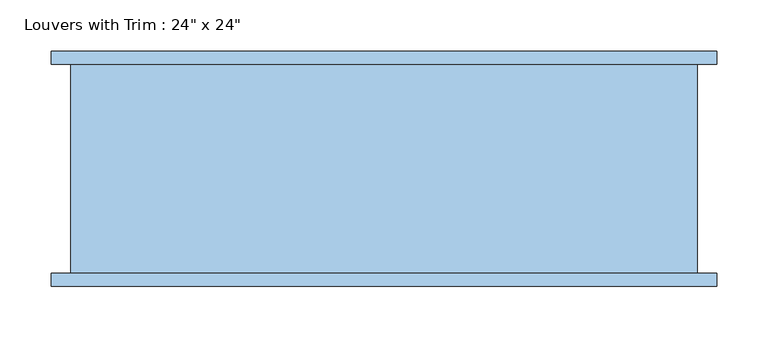
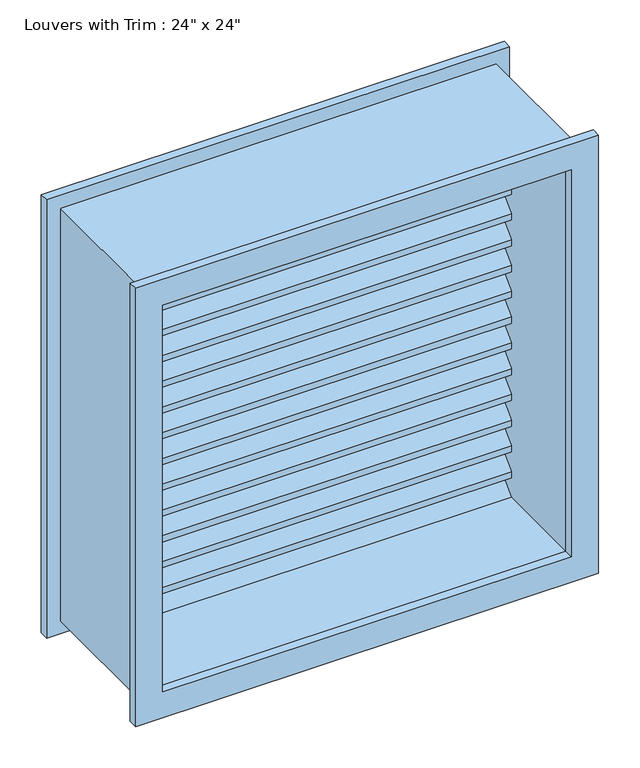
"""IFC4 building model written with IfcOpenShell, lengths in millimetres: window geometry."""

from ifc_helpers import new_model, si_unit, frame, origin, place, context, project, spatial, polyline, outline, extrude, source, transform, mapped, element, save


def window_0038ecf3(model_context):
    return source(origin(), model_context, "Body", "SweptSolid", [
        extrude(outline(polyline([(1543.05, -323.85), (895.35, -323.85), (895.35, 323.85), (1543.05, 323.85), (1543.05, -323.85)]), holes=[polyline([(1504.95, -285.75), (1504.95, 285.75), (933.45, 285.75), (933.45, -285.75), (1504.95, -285.75)])]), frame((0.0, 95.25, 0.0), z_axis=(0.0, 1.0, 0.0), x_axis=(0.0, 0.0, 1.0)), (0.0, 0.0, 1.0), 12.7),
        extrude(outline(polyline([(1543.05, 323.85), (1543.05, -323.85), (895.35, -323.85), (895.35, 323.85), (1543.05, 323.85)]), holes=[polyline([(1504.95, 285.75), (933.45, 285.75), (933.45, -285.75), (1504.95, -285.75), (1504.95, 285.75)])]), frame((0.0, -120.65, 0.0), z_axis=(0.0, 1.0, 0.0), x_axis=(0.0, 0.0, 1.0)), (0.0, 0.0, 1.0), 12.7),
        extrude(outline(polyline([(1524.0, 304.8), (1524.0, -304.8), (914.4, -304.8), (914.4, 304.8), (1524.0, 304.8)]), holes=[polyline([(1504.95, 285.75), (933.45, 285.75), (933.45, -285.75), (1504.95, -285.75), (1504.95, 285.75)])]), frame((0.0, -107.95, 0.0), z_axis=(0.0, 1.0, 0.0), x_axis=(0.0, 0.0, 1.0)), (0.0, 0.0, 1.0), 203.2),
        extrude(outline(polyline([(59.3289755, 969.3710245), (95.25, 933.45), (86.2697439, 933.45), (59.3289755, 960.3907684), (32.3882072, 933.45), (23.407951, 933.45), (59.3289755, 969.3710245)])), frame((-285.75, 0.0, 0.0), z_axis=(1.0, 0.0, 0.0), x_axis=(0.0, 1.0, 0.0)), (0.0, 0.0, 1.0), 571.5),
        extrude(outline(polyline([(59.3289755, 1007.4710245), (95.25, 971.55), (95.25, 962.5697439), (59.3289755, 998.4907684), (23.407951, 962.5697439), (23.407951, 971.55), (59.3289755, 1007.4710245)])), frame((-285.75, 0.0, 0.0), z_axis=(1.0, 0.0, 0.0), x_axis=(0.0, 1.0, 0.0)), (0.0, 0.0, 1.0), 571.5),
        extrude(outline(polyline([(59.3289755, 1045.5710245), (95.25, 1009.65), (95.25, 1000.6697439), (59.3289755, 1036.5907684), (23.407951, 1000.6697439), (23.407951, 1009.65), (59.3289755, 1045.5710245)])), frame((-285.75, 0.0, 0.0), z_axis=(1.0, 0.0, 0.0), x_axis=(0.0, 1.0, 0.0)), (0.0, 0.0, 1.0), 571.5),
        extrude(outline(polyline([(59.3289755, 1083.6710245), (95.25, 1047.75), (95.25, 1038.7697439), (59.3289755, 1074.6907684), (23.407951, 1038.7697439), (23.407951, 1047.75), (59.3289755, 1083.6710245)])), frame((-285.75, 0.0, 0.0), z_axis=(1.0, 0.0, 0.0), x_axis=(0.0, 1.0, 0.0)), (0.0, 0.0, 1.0), 571.5),
        extrude(outline(polyline([(59.3289755, 1121.7710245), (95.25, 1085.85), (95.25, 1076.8697439), (59.3289755, 1112.7907684), (23.407951, 1076.8697439), (23.407951, 1085.85), (59.3289755, 1121.7710245)])), frame((-285.75, 0.0, 0.0), z_axis=(1.0, 0.0, 0.0), x_axis=(0.0, 1.0, 0.0)), (0.0, 0.0, 1.0), 571.5),
        extrude(outline(polyline([(59.3289755, 1159.8710245), (95.25, 1123.95), (95.25, 1114.9697439), (59.3289755, 1150.8907684), (23.407951, 1114.9697439), (23.407951, 1123.95), (59.3289755, 1159.8710245)])), frame((-285.75, 0.0, 0.0), z_axis=(1.0, 0.0, 0.0), x_axis=(0.0, 1.0, 0.0)), (0.0, 0.0, 1.0), 571.5),
        extrude(outline(polyline([(59.3289755, 1197.9710245), (95.25, 1162.05), (95.25, 1153.0697439), (59.3289755, 1188.9907684), (23.407951, 1153.0697439), (23.407951, 1162.05), (59.3289755, 1197.9710245)])), frame((-285.75, 0.0, 0.0), z_axis=(1.0, 0.0, 0.0), x_axis=(0.0, 1.0, 0.0)), (0.0, 0.0, 1.0), 571.5),
        extrude(outline(polyline([(59.3289755, 1236.0710245), (95.25, 1200.15), (95.25, 1191.1697439), (59.3289755, 1227.0907684), (23.407951, 1191.1697439), (23.407951, 1200.15), (59.3289755, 1236.0710245)])), frame((-285.75, 0.0, 0.0), z_axis=(1.0, 0.0, 0.0), x_axis=(0.0, 1.0, 0.0)), (0.0, 0.0, 1.0), 571.5),
        extrude(outline(polyline([(59.3289755, 1274.1710245), (95.25, 1238.25), (95.25, 1229.2697439), (59.3289755, 1265.1907684), (23.407951, 1229.2697439), (23.407951, 1238.25), (59.3289755, 1274.1710245)])), frame((-285.75, 0.0, 0.0), z_axis=(1.0, 0.0, 0.0), x_axis=(0.0, 1.0, 0.0)), (0.0, 0.0, 1.0), 571.5),
        extrude(outline(polyline([(59.3289755, 1312.2710245), (95.25, 1276.35), (95.25, 1267.3697439), (59.3289755, 1303.2907684), (23.407951, 1267.3697439), (23.407951, 1276.35), (59.3289755, 1312.2710245)])), frame((-285.75, 0.0, 0.0), z_axis=(1.0, 0.0, 0.0), x_axis=(0.0, 1.0, 0.0)), (0.0, 0.0, 1.0), 571.5),
        extrude(outline(polyline([(59.3289755, 1350.3710245), (95.25, 1314.45), (95.25, 1305.4697439), (59.3289755, 1341.3907684), (23.407951, 1305.4697439), (23.407951, 1314.45), (59.3289755, 1350.3710245)])), frame((-285.75, 0.0, 0.0), z_axis=(1.0, 0.0, 0.0), x_axis=(0.0, 1.0, 0.0)), (0.0, 0.0, 1.0), 571.5),
        extrude(outline(polyline([(59.3289755, 1388.4710245), (95.25, 1352.55), (95.25, 1343.5697439), (59.3289755, 1379.4907684), (23.407951, 1343.5697439), (23.407951, 1352.55), (59.3289755, 1388.4710245)])), frame((-285.75, 0.0, 0.0), z_axis=(1.0, 0.0, 0.0), x_axis=(0.0, 1.0, 0.0)), (0.0, 0.0, 1.0), 571.5),
        extrude(outline(polyline([(59.3289755, 1426.5710245), (95.25, 1390.65), (95.25, 1381.6697439), (59.3289755, 1417.5907684), (23.407951, 1381.6697439), (23.407951, 1390.65), (59.3289755, 1426.5710245)])), frame((-285.75, 0.0, 0.0), z_axis=(1.0, 0.0, 0.0), x_axis=(0.0, 1.0, 0.0)), (0.0, 0.0, 1.0), 571.5),
        extrude(outline(polyline([(59.3289755, 1464.6710245), (95.25, 1428.75), (95.25, 1419.7697439), (59.3289755, 1455.6907684), (23.407951, 1419.7697439), (23.407951, 1428.75), (59.3289755, 1464.6710245)])), frame((-285.75, 0.0, 0.0), z_axis=(1.0, 0.0, 0.0), x_axis=(0.0, 1.0, 0.0)), (0.0, 0.0, 1.0), 571.5),
        extrude(outline(polyline([(59.3289755, 1502.7710245), (95.25, 1466.85), (95.25, 1457.8697439), (59.3289755, 1493.7907684), (23.407951, 1457.8697439), (23.407951, 1466.85), (59.3289755, 1502.7710245)])), frame((-285.75, 0.0, 0.0), z_axis=(1.0, 0.0, 0.0), x_axis=(0.0, 1.0, 0.0)), (0.0, 0.0, 1.0), 571.5),
    ])


if __name__ == "__main__":
    model = new_model("IFC4")
    model_context = context("Model", 3, world=origin())
    ifc_project = project(units=[si_unit("LENGTHUNIT", "METRE", prefix="MILLI")], contexts=[model_context])
    site = spatial("IfcSite", under=ifc_project)
    building = spatial("IfcBuilding", under=site)
    placement = place(None, origin())
    window_shape = window_0038ecf3(model_context)
    element("IfcWindow", 1, ObjectType="Louvers with Trim : 24\" x 24\"", at=placement, inside=building, context=model_context, shape_type="MappedRepresentation", body=[
        mapped(window_shape, transform((0.0, 0.0, 0.0), x_axis=(1.0, 0.0, 0.0), y_axis=(0.0, 1.0, 0.0), z_axis=(0.0, 0.0, 1.0))),
    ])
    save(model, "model.ifc")

# Revit data of these elements
# Type "Louvers with Trim : 24\" x 24\""
#   Type Mark = "10"
#   Construction Type Id = "GSP4R"
#   Assembly Code = "B20"
#   Analytic Construction = "1/8 in Pilkington single glazing"
#   Visual Light Transmittance = 0.9
#   Solar Heat Gain Coefficient = 0.78
#   Heat Transfer Coefficient (U) = 0.6496 BTU/(h·ft²·°F)
#   Default Sill Height = 3' - 0"
#   Trim Projection - Ext. = 0' - 0 1/2"
#   Trim Projection - Int. = 0' - 0 1/2"
#   Trim Width - Exterior = 0' - 1 1/2"
#   Trim Width - Interior = 0' - 1 1/2"
#   Width = 2' - 0"
#   Define Thermal Properties by = 1
#   Frame Material = Birch
#   Louver Material = Birch
#   Trim Exterior Material = Birch
#   Trim Interior Material = Birch
#   Wall Closure = (empty or 0)
# Element 1 (IfcWindow, "Louvers with Trim : 24\" x 24\"")
#   Materials on its faces: "Birch"
# Materials
#   "Birch": class "Wood", colour RGB 224 178 126, transparency 0, Description = "Betula Alleghaniensis", Cost = 0
